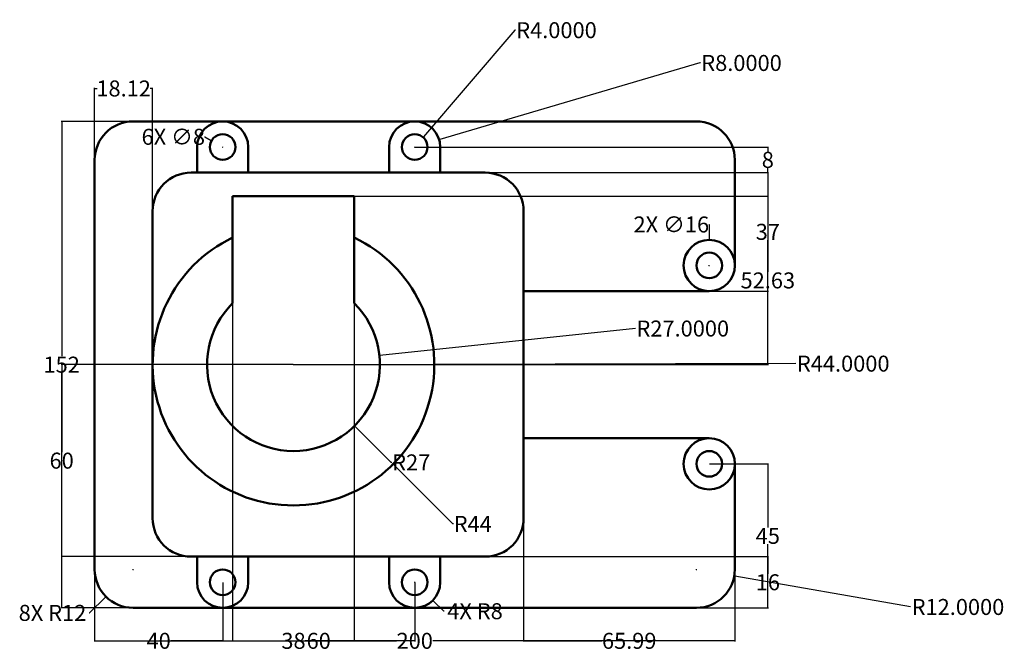
# Model space of a CAD drawing. Units: inches. Extents: x 381008 to 381315, y 259803 to 260000.
import ezdxf

# ---------------------------------------------------------------- set-up
doc = ezdxf.new("R2010")
doc.units = ezdxf.units.IN
doc.header["$MEASUREMENT"] = 0
doc.layers.add('M-DIMS', color=2, linetype='Continuous', lineweight=25)
doc.layers.add('M-OUTL', color=7, linetype='Continuous', lineweight=50)
doc.styles.get("Standard").update_dxf_attribs({"font": 'arial.ttf'})
doc.dimstyles.get("Standard").update_dxf_attribs({"dimtxt": 5, "dimasz": 0.18, "dimexe": 0.18, "dimexo": 0.0625, "dimgap": 0.09, "dimtad": 0, "dimtih": 1, "dimtoh": 1, "dimdec": 4, "dimzin": 0, "dimdsep": 46, "dimtxsty": 'Standard', "dimcen": 0.09, "dimadec": 0, "dimazin": 0, "dimtfac": 1, "dimtdec": 4, "dimtofl": 0, "dimtmove": 0, "dimatfit": 3, "dimfxl": 1, "dimtolj": 1, "dimtzin": 0, "dimarcsym": 0})

# ---------------------------------------------------------------- blocks, each defined once
blk = doc.blocks.new('*D1')
at = {"layer": 'Defpoints', "color": 0, "transparency": 16777216}
for p in [(381133.58, 259963.48), (381130.98, 259960.44)]:
    blk.add_point(p, dxfattribs=at)
at = {"layer": 'M-DIMS', "color": 0, "lineweight": -2, "transparency": 16777216}
for p, q in [((381162.25, 259996.96), (381133.7, 259963.62)), ((381162.43, 259996.96), (381162.25, 259996.96)), ((381130.89, 259960.44), (381131.07, 259960.44)), ((381130.98, 259960.35), (381130.98, 259960.53))]:
    blk.add_line(p, q, dxfattribs=at)
at = {"layer": 'M-DIMS', "color": 0, "transparency": 16777216}
blk.add_solid([(381133.68, 259963.64), (381133.72, 259963.6), (381133.58, 259963.48)], dxfattribs=at)
at = {"layer": 'M-DIMS', "color": 0, "transparency": 16777216, "insert": (381175.28, 259996.96), "char_height": 5, "attachment_point": 5}
blk.add_mtext('\\A1;R4.0000', dxfattribs=at)
blk = doc.blocks.new('*D2')
at = {"layer": 'Defpoints', "color": 0, "transparency": 16777216}
for p in [(381130.98, 259960.44), (381138.66, 259962.71)]:
    blk.add_point(p, dxfattribs=at)
at = {"layer": 'M-DIMS', "color": 0, "lineweight": -2, "transparency": 16777216}
for p, q in [((381220.06, 259986.72), (381138.83, 259962.76)), ((381220.24, 259986.72), (381220.06, 259986.72)), ((381130.89, 259960.44), (381131.07, 259960.44)), ((381130.98, 259960.35), (381130.98, 259960.53))]:
    blk.add_line(p, q, dxfattribs=at)
at = {"layer": 'M-DIMS', "color": 0, "transparency": 16777216}
blk.add_solid([(381138.82, 259962.79), (381138.84, 259962.73), (381138.66, 259962.71)], dxfattribs=at)
at = {"layer": 'M-DIMS', "color": 0, "transparency": 16777216, "insert": (381233.09, 259986.72), "char_height": 5, "attachment_point": 5}
blk.add_mtext('\\A1;R8.0000', dxfattribs=at)
blk = doc.blocks.new('*D3')
at = {"layer": 'Defpoints', "color": 0, "transparency": 16777216}
for p in [(381218.99, 259828.44), (381230.81, 259826.37)]:
    blk.add_point(p, dxfattribs=at)
at = {"layer": 'M-DIMS', "color": 0, "lineweight": -2, "transparency": 16777216}
for p, q in [((381218.9, 259828.44), (381219.08, 259828.44)), ((381218.99, 259828.35), (381218.99, 259828.53)), ((381285.92, 259816.72), (381230.98, 259826.34))]:
    blk.add_line(p, q, dxfattribs=at)
at = {"layer": 'M-DIMS', "color": 0, "transparency": 16777216}
blk.add_solid([(381230.99, 259826.37), (381230.98, 259826.31), (381230.81, 259826.37)], dxfattribs=at)
at = {"layer": 'M-DIMS', "color": 0, "transparency": 16777216, "insert": (381300.71, 259816.72), "char_height": 5, "attachment_point": 5}
blk.add_mtext('\\A1;R12.0000', dxfattribs=at)
blk = doc.blocks.new('*D4')
at = {"layer": 'Defpoints', "color": 0, "transparency": 16777216}
for p in [(381093.1, 259892.44), (381137.1, 259892.53)]:
    blk.add_point(p, dxfattribs=at)
at = {"layer": 'M-DIMS', "color": 0, "lineweight": -2, "transparency": 16777216}
for p, q in [((381250.06, 259892.76), (381137.28, 259892.53)), ((381093.01, 259892.44), (381093.19, 259892.44)), ((381093.1, 259892.35), (381093.1, 259892.53))]:
    blk.add_line(p, q, dxfattribs=at)
at = {"layer": 'M-DIMS', "color": 0, "transparency": 16777216}
blk.add_solid([(381137.28, 259892.56), (381137.28, 259892.5), (381137.1, 259892.53)], dxfattribs=at)
at = {"layer": 'M-DIMS', "color": 0, "transparency": 16777216, "insert": (381264.86, 259892.76), "char_height": 5, "attachment_point": 5}
blk.add_mtext('\\A1;R44.0000', dxfattribs=at)
blk = doc.blocks.new('*D5')
at = {"layer": 'Defpoints', "color": 0, "transparency": 16777216}
for p in [(381119.95, 259895.28), (381093.1, 259892.44)]:
    blk.add_point(p, dxfattribs=at)
at = {"layer": 'M-DIMS', "color": 0, "lineweight": -2, "transparency": 16777216}
for p, q in [((381199.94, 259903.73), (381120.13, 259895.3)), ((381093.01, 259892.44), (381093.19, 259892.44)), ((381093.1, 259892.35), (381093.1, 259892.53))]:
    blk.add_line(p, q, dxfattribs=at)
at = {"layer": 'M-DIMS', "color": 0, "transparency": 16777216}
blk.add_solid([(381120.13, 259895.33), (381120.13, 259895.27), (381119.95, 259895.28)], dxfattribs=at)
at = {"layer": 'M-DIMS', "color": 0, "transparency": 16777216, "insert": (381214.73, 259903.73), "char_height": 5, "attachment_point": 5}
blk.add_mtext('\\A1;R27.0000', dxfattribs=at)
blk = doc.blocks.new('MOUNTING-LUG')
for p, q in [((-8, 0), (-8, -8)), ((8, 0), (8, -8))]:
    blk.add_line(p, q)
blk.add_circle((0, 0), 4)
blk.add_arc((0, 0), 8, 0, 180)
blk = doc.blocks.new('CONCENTRIC-MOUNT-HOLE')
for radius in [8, 4]:
    blk.add_circle((0, 0), radius)
blk = doc.blocks.new('*D8')
at = {"layer": 'Defpoints', "color": 0, "transparency": 16777216}
for p in [(381030.98, 259828.44), (381230.99, 259828.44), (381230.99, 259806.14)]:
    blk.add_point(p, dxfattribs=at)
at = {"layer": 'M-DIMS', "color": 0, "lineweight": -2, "transparency": 16777216}
for p, q in [((381030.98, 259828.38), (381030.98, 259805.96)), ((381230.99, 259828.38), (381230.99, 259805.96)), ((381031.16, 259806.14), (381125.34, 259806.14)), ((381230.81, 259806.14), (381136.63, 259806.14))]:
    blk.add_line(p, q, dxfattribs=at)
at = {"layer": 'M-DIMS', "color": 0, "transparency": 16777216}
for points in [[(381031.16, 259806.17), (381031.16, 259806.11), (381030.98, 259806.14)], [(381230.81, 259806.17), (381230.81, 259806.11), (381230.99, 259806.14)]]:
    blk.add_solid(points, dxfattribs=at)
at = {"layer": 'M-DIMS', "color": 0, "transparency": 16777216, "insert": (381130.98, 259806.14), "char_height": 5, "attachment_point": 5}
blk.add_mtext('\\A1;200', dxfattribs=at)
blk = doc.blocks.new('*D9')
at = {"layer": 'Defpoints', "color": 0, "transparency": 16777216}
for p in [(381020.68, 259968.44), (381042.98, 259968.44), (381042.98, 259816.44)]:
    blk.add_point(p, dxfattribs=at)
at = {"layer": 'M-DIMS', "color": 0, "lineweight": -2, "transparency": 16777216}
for p, q in [((381042.92, 259968.44), (381020.5, 259968.44)), ((381020.68, 259968.26), (381020.68, 259895.09)), ((381020.68, 259816.62), (381020.68, 259889.8)), ((381042.92, 259816.44), (381020.5, 259816.44))]:
    blk.add_line(p, q, dxfattribs=at)
at = {"layer": 'M-DIMS', "color": 0, "transparency": 16777216}
for points in [[(381020.65, 259968.26), (381020.71, 259968.26), (381020.68, 259968.44)], [(381020.65, 259816.62), (381020.71, 259816.62), (381020.68, 259816.44)]]:
    blk.add_solid(points, dxfattribs=at)
at = {"layer": 'M-DIMS', "color": 0, "transparency": 16777216, "insert": (381020.68, 259892.44), "char_height": 5, "attachment_point": 5}
blk.add_mtext('\\A1;152', dxfattribs=at)
blk = doc.blocks.new('*D10')
at = {"layer": 'Defpoints', "color": 0, "transparency": 16777216}
for p in [(381030.98, 259828.44), (381070.98, 259824.44), (381070.98, 259806.14)]:
    blk.add_point(p, dxfattribs=at)
at = {"layer": 'M-DIMS', "color": 0, "lineweight": -2, "transparency": 16777216}
for p, q in [((381030.98, 259828.38), (381030.98, 259805.96)), ((381070.98, 259824.38), (381070.98, 259805.96)), ((381031.16, 259806.14), (381047.22, 259806.14)), ((381070.8, 259806.14), (381054.75, 259806.14))]:
    blk.add_line(p, q, dxfattribs=at)
at = {"layer": 'M-DIMS', "color": 0, "transparency": 16777216}
for points in [[(381031.16, 259806.17), (381031.16, 259806.11), (381030.98, 259806.14)], [(381070.8, 259806.17), (381070.8, 259806.11), (381070.98, 259806.14)]]:
    blk.add_solid(points, dxfattribs=at)
at = {"layer": 'M-DIMS', "color": 0, "transparency": 16777216, "insert": (381050.98, 259806.14), "char_height": 5, "attachment_point": 5}
blk.add_mtext('\\A1;40', dxfattribs=at)
blk = doc.blocks.new('*D11')
at = {"layer": 'Defpoints', "color": 0, "transparency": 16777216}
for p in [(381070.98, 259824.44), (381130.98, 259824.44), (381130.98, 259806.14)]:
    blk.add_point(p, dxfattribs=at)
at = {"layer": 'M-DIMS', "color": 0, "lineweight": -2, "transparency": 16777216}
for p, q in [((381070.98, 259824.38), (381070.98, 259805.96)), ((381130.98, 259824.38), (381130.98, 259805.96)), ((381071.16, 259806.14), (381097.31, 259806.14)), ((381130.8, 259806.14), (381104.66, 259806.14))]:
    blk.add_line(p, q, dxfattribs=at)
at = {"layer": 'M-DIMS', "color": 0, "transparency": 16777216}
for points in [[(381071.16, 259806.17), (381071.16, 259806.11), (381070.98, 259806.14)], [(381130.8, 259806.17), (381130.8, 259806.11), (381130.98, 259806.14)]]:
    blk.add_solid(points, dxfattribs=at)
at = {"layer": 'M-DIMS', "color": 0, "transparency": 16777216, "insert": (381100.98, 259806.14), "char_height": 5, "attachment_point": 5}
blk.add_mtext('\\A1;60', dxfattribs=at)
blk = doc.blocks.new('*D12')
at = {"layer": 'Defpoints', "color": 0, "transparency": 16777216}
for p in [(381049.1, 259978.74), (381030.98, 259956.44), (381049.1, 259940.44)]:
    blk.add_point(p, dxfattribs=at)
at = {"layer": 'M-DIMS', "color": 0, "lineweight": -2, "transparency": 16777216}
for p, q in [((381030.98, 259956.51), (381030.98, 259978.92)), ((381049.1, 259940.51), (381049.1, 259978.92)), ((381031.16, 259978.74), (381031.78, 259978.74)), ((381048.92, 259978.74), (381048.31, 259978.74))]:
    blk.add_line(p, q, dxfattribs=at)
at = {"layer": 'M-DIMS', "color": 0, "transparency": 16777216}
for points in [[(381031.16, 259978.77), (381031.16, 259978.71), (381030.98, 259978.74)], [(381048.92, 259978.77), (381048.92, 259978.71), (381049.1, 259978.74)]]:
    blk.add_solid(points, dxfattribs=at)
at = {"layer": 'M-DIMS', "color": 0, "transparency": 16777216, "insert": (381040.04, 259978.74), "char_height": 5, "attachment_point": 5}
blk.add_mtext('\\A1;18.12', dxfattribs=at)
blk = doc.blocks.new('*D13')
at = {"layer": 'Defpoints', "color": 0, "transparency": 16777216}
for p in [(381165, 259844.44), (381230.99, 259828.44), (381230.99, 259806.14)]:
    blk.add_point(p, dxfattribs=at)
at = {"layer": 'M-DIMS', "color": 0, "lineweight": -2, "transparency": 16777216}
for p, q in [((381165, 259844.38), (381165, 259805.96)), ((381230.99, 259828.38), (381230.99, 259805.96)), ((381165.18, 259806.14), (381189.45, 259806.14)), ((381230.81, 259806.14), (381206.54, 259806.14))]:
    blk.add_line(p, q, dxfattribs=at)
at = {"layer": 'M-DIMS', "color": 0, "transparency": 16777216}
for points in [[(381165.18, 259806.17), (381165.18, 259806.11), (381165, 259806.14)], [(381230.81, 259806.17), (381230.81, 259806.11), (381230.99, 259806.14)]]:
    blk.add_solid(points, dxfattribs=at)
at = {"layer": 'M-DIMS', "color": 0, "transparency": 16777216, "insert": (381197.99, 259806.14), "char_height": 5, "attachment_point": 5}
blk.add_mtext('\\A1;65.99', dxfattribs=at)
blk = doc.blocks.new('*D14')
at = {"layer": 'Defpoints', "color": 0, "transparency": 16777216}
for p in [(381020.68, 259892.44), (381093.1, 259892.44), (381061.1, 259832.44)]:
    blk.add_point(p, dxfattribs=at)
at = {"layer": 'M-DIMS', "color": 0, "lineweight": -2, "transparency": 16777216}
for p, q in [((381093.04, 259892.44), (381020.5, 259892.44)), ((381020.68, 259892.26), (381020.68, 259865.09)), ((381020.68, 259832.62), (381020.68, 259859.8)), ((381061.04, 259832.44), (381020.5, 259832.44))]:
    blk.add_line(p, q, dxfattribs=at)
at = {"layer": 'M-DIMS', "color": 0, "transparency": 16777216}
for points in [[(381020.65, 259892.26), (381020.71, 259892.26), (381020.68, 259892.44)], [(381020.65, 259832.62), (381020.71, 259832.62), (381020.68, 259832.44)]]:
    blk.add_solid(points, dxfattribs=at)
at = {"layer": 'M-DIMS', "color": 0, "transparency": 16777216, "insert": (381020.68, 259862.44), "char_height": 5, "attachment_point": 5}
blk.add_mtext('\\A1;60', dxfattribs=at)
blk = doc.blocks.new('*D15')
at = {"layer": 'Defpoints', "color": 0, "transparency": 16777216}
for p in [(381130.98, 259960.44), (381153, 259952.44), (381241.3, 259952.44)]:
    blk.add_point(p, dxfattribs=at)
at = {"layer": 'M-DIMS', "color": 0, "lineweight": -2, "transparency": 16777216}
for p, q in [((381131.04, 259960.44), (381241.48, 259960.44)), ((381241.3, 259960.26), (381241.3, 259959.09)), ((381153.06, 259952.44), (381241.48, 259952.44)), ((381241.3, 259952.62), (381241.3, 259953.8))]:
    blk.add_line(p, q, dxfattribs=at)
at = {"layer": 'M-DIMS', "color": 0, "transparency": 16777216}
for points in [[(381241.27, 259960.26), (381241.33, 259960.26), (381241.3, 259960.44)], [(381241.27, 259952.62), (381241.33, 259952.62), (381241.3, 259952.44)]]:
    blk.add_solid(points, dxfattribs=at)
at = {"layer": 'M-DIMS', "color": 0, "transparency": 16777216, "insert": (381241.3, 259956.44), "char_height": 5, "attachment_point": 5}
blk.add_mtext('\\A1;8', dxfattribs=at)
blk = doc.blocks.new('*D16')
at = {"layer": 'Defpoints', "color": 0, "transparency": 16777216}
for p in [(381153, 259832.44), (381241.3, 259832.44), (381218.99, 259816.44)]:
    blk.add_point(p, dxfattribs=at)
at = {"layer": 'M-DIMS', "color": 0, "lineweight": -2, "transparency": 16777216}
for p, q in [((381153.06, 259832.44), (381241.48, 259832.44)), ((381241.3, 259832.26), (381241.3, 259827.09)), ((381241.3, 259816.62), (381241.3, 259821.8)), ((381219.05, 259816.44), (381241.48, 259816.44))]:
    blk.add_line(p, q, dxfattribs=at)
at = {"layer": 'M-DIMS', "color": 0, "transparency": 16777216}
for points in [[(381241.27, 259832.26), (381241.33, 259832.26), (381241.3, 259832.44)], [(381241.27, 259816.62), (381241.33, 259816.62), (381241.3, 259816.44)]]:
    blk.add_solid(points, dxfattribs=at)
at = {"layer": 'M-DIMS', "color": 0, "transparency": 16777216, "insert": (381241.3, 259824.44), "char_height": 5, "attachment_point": 5}
blk.add_mtext('\\A1;16', dxfattribs=at)
blk = doc.blocks.new('*D17')
at = {"layer": 'Defpoints', "color": 0, "transparency": 16777216}
for p in [(381153, 259952.44), (381241.3, 259952.44), (381165, 259915.44)]:
    blk.add_point(p, dxfattribs=at)
at = {"layer": 'M-DIMS', "color": 0, "lineweight": -2, "transparency": 16777216}
for p, q in [((381153.06, 259952.44), (381241.48, 259952.44)), ((381241.3, 259952.26), (381241.3, 259936.59)), ((381241.3, 259915.62), (381241.3, 259931.3)), ((381165.06, 259915.44), (381241.48, 259915.44))]:
    blk.add_line(p, q, dxfattribs=at)
at = {"layer": 'M-DIMS', "color": 0, "transparency": 16777216}
for points in [[(381241.27, 259952.26), (381241.33, 259952.26), (381241.3, 259952.44)], [(381241.27, 259915.62), (381241.33, 259915.62), (381241.3, 259915.44)]]:
    blk.add_solid(points, dxfattribs=at)
at = {"layer": 'M-DIMS', "color": 0, "transparency": 16777216, "insert": (381241.3, 259933.94), "char_height": 5, "attachment_point": 5}
blk.add_mtext('\\A1;37', dxfattribs=at)
blk = doc.blocks.new('*D18')
at = {"layer": 'Defpoints', "color": 0, "transparency": 16777216}
for p in [(381223.000594, 259861.442622), (381241.300594, 259861.442622), (381218.986961, 259816.442622)]:
    blk.add_point(p, dxfattribs=at)
at = {"layer": 'M-DIMS', "color": 0, "lineweight": -2, "transparency": 16777216}
for p, q in [((381223.063094, 259861.442622), (381241.480594, 259861.442622)), ((381241.300594, 259861.262622), (381241.300594, 259841.575255)), ((381241.300594, 259816.622622), (381241.300594, 259836.309989)), ((381219.049461, 259816.442622), (381241.480594, 259816.442622))]:
    blk.add_line(p, q, dxfattribs=at)
at = {"layer": 'M-DIMS', "color": 0, "transparency": 16777216}
for points in [[(381241.270594, 259861.262622), (381241.330594, 259861.262622), (381241.300594, 259861.442622)], [(381241.270594, 259816.622622), (381241.330594, 259816.622622), (381241.300594, 259816.442622)]]:
    blk.add_solid(points, dxfattribs=at)
at = {"layer": 'M-DIMS', "color": 0, "transparency": 16777216, "insert": (381241.300594, 259838.942622), "char_height": 5, "attachment_point": 5}
blk.add_mtext('\\A1;45', dxfattribs=at)
blk = doc.blocks.new('*D19')
at = {"layer": 'Defpoints', "color": 0, "transparency": 16777216}
for p in [(381074.1, 259945.07), (381112.1, 259945.07), (381112.1, 259806.14)]:
    blk.add_point(p, dxfattribs=at)
at = {"layer": 'M-DIMS', "color": 0, "lineweight": -2, "transparency": 16777216}
for p, q in [((381074.1, 259945.01), (381074.1, 259805.96)), ((381112.1, 259945.01), (381112.1, 259805.96)), ((381074.28, 259806.14), (381089.43, 259806.14)), ((381111.92, 259806.14), (381096.77, 259806.14))]:
    blk.add_line(p, q, dxfattribs=at)
at = {"layer": 'M-DIMS', "color": 0, "transparency": 16777216}
for points in [[(381074.28, 259806.17), (381074.28, 259806.11), (381074.1, 259806.14)], [(381111.92, 259806.17), (381111.92, 259806.11), (381112.1, 259806.14)]]:
    blk.add_solid(points, dxfattribs=at)
at = {"layer": 'M-DIMS', "color": 0, "transparency": 16777216, "insert": (381093.1, 259806.14), "char_height": 5, "attachment_point": 5}
blk.add_mtext('\\A1;38', dxfattribs=at)
blk = doc.blocks.new('*D20')
at = {"layer": 'Defpoints', "color": 0, "transparency": 16777216}
for p in [(381112.1, 259945.07), (381241.3, 259945.07), (381093.1, 259892.44)]:
    blk.add_point(p, dxfattribs=at)
at = {"layer": 'M-DIMS', "color": 0, "lineweight": -2, "transparency": 16777216}
for p, q in [((381112.16, 259945.07), (381241.48, 259945.07)), ((381241.3, 259944.89), (381241.3, 259921.4)), ((381241.3, 259892.62), (381241.3, 259916.11)), ((381093.16, 259892.44), (381241.48, 259892.44))]:
    blk.add_line(p, q, dxfattribs=at)
at = {"layer": 'M-DIMS', "color": 0, "transparency": 16777216}
for points in [[(381241.27, 259944.89), (381241.33, 259944.89), (381241.3, 259945.07)], [(381241.27, 259892.62), (381241.33, 259892.62), (381241.3, 259892.44)]]:
    blk.add_solid(points, dxfattribs=at)
at = {"layer": 'M-DIMS', "color": 0, "transparency": 16777216, "insert": (381241.3, 259918.76), "char_height": 5, "attachment_point": 5}
blk.add_mtext('\\A1;52.63', dxfattribs=at)
blk = doc.blocks.new('*D21')
at = {"layer": 'Defpoints', "color": 0, "transparency": 16777216}
for p in [(381042.98, 259828.44), (381034.5, 259819.96)]:
    blk.add_point(p, dxfattribs=at)
at = {"layer": 'M-DIMS', "color": 0, "lineweight": -2, "transparency": 16777216}
for p, q in [((381042.89, 259828.44), (381043.07, 259828.44)), ((381042.98, 259828.35), (381042.98, 259828.53)), ((381029.41, 259814.87), (381034.37, 259819.83)), ((381029.23, 259814.87), (381029.41, 259814.87))]:
    blk.add_line(p, q, dxfattribs=at)
at = {"layer": 'M-DIMS', "color": 0, "transparency": 16777216}
blk.add_solid([(381034.35, 259819.85), (381034.39, 259819.81), (381034.5, 259819.96)], dxfattribs=at)
at = {"layer": 'M-DIMS', "color": 0, "transparency": 16777216, "insert": (381017.81, 259814.87), "char_height": 5, "attachment_point": 5}
blk.add_mtext('\\A1;8X R12', dxfattribs=at)
blk = doc.blocks.new('*D22')
at = {"layer": 'Defpoints', "color": 0, "transparency": 16777216}
for p in [(381130.98, 259824.44), (381136.64, 259818.79)]:
    blk.add_point(p, dxfattribs=at)
at = {"layer": 'M-DIMS', "color": 0, "lineweight": -2, "transparency": 16777216}
for p, q in [((381130.89, 259824.44), (381131.07, 259824.44)), ((381130.98, 259824.35), (381130.98, 259824.53)), ((381140.04, 259815.4), (381136.77, 259818.66)), ((381140.22, 259815.4), (381140.04, 259815.4))]:
    blk.add_line(p, q, dxfattribs=at)
at = {"layer": 'M-DIMS', "color": 0, "transparency": 16777216}
blk.add_solid([(381136.79, 259818.68), (381136.75, 259818.64), (381136.64, 259818.79)], dxfattribs=at)
at = {"layer": 'M-DIMS', "color": 0, "transparency": 16777216, "insert": (381149.82, 259815.4), "char_height": 5, "attachment_point": 5}
blk.add_mtext('\\A1;4X R8', dxfattribs=at)
blk = doc.blocks.new('*D23')
at = {"layer": 'Defpoints', "color": 0, "transparency": 16777216}
for p in [(381067.52, 259962.44), (381074.45, 259958.44)]:
    blk.add_point(p, dxfattribs=at)
at = {"layer": 'M-DIMS', "color": 0, "lineweight": -2, "transparency": 16777216}
for p, q in [((381065.26, 259963.64), (381065.44, 259963.64)), ((381065.44, 259963.64), (381067.36, 259962.53)), ((381070.89, 259960.44), (381071.07, 259960.44)), ((381070.98, 259960.35), (381070.98, 259960.53))]:
    blk.add_line(p, q, dxfattribs=at)
at = {"layer": 'M-DIMS', "color": 0, "transparency": 16777216}
blk.add_solid([(381067.38, 259962.56), (381067.35, 259962.51), (381067.52, 259962.44)], dxfattribs=at)
at = {"layer": 'M-DIMS', "color": 0, "transparency": 16777216, "insert": (381055.55, 259963.64), "char_height": 5, "attachment_point": 5}
blk.add_mtext('\\A1;6X ∅8', dxfattribs=at)
blk = doc.blocks.new('*D24')
at = {"layer": 'Defpoints', "color": 0, "transparency": 16777216}
for p in [(381223, 259931.44), (381223, 259915.44)]:
    blk.add_point(p, dxfattribs=at)
at = {"layer": 'M-DIMS', "color": 0, "lineweight": -2, "transparency": 16777216}
for p, q in [((381222.82, 259936.24), (381223, 259936.24)), ((381223, 259936.24), (381223, 259931.62)), ((381222.91, 259923.44), (381223.09, 259923.44)), ((381223, 259923.35), (381223, 259923.53))]:
    blk.add_line(p, q, dxfattribs=at)
at = {"layer": 'M-DIMS', "color": 0, "transparency": 16777216}
blk.add_solid([(381223.03, 259931.62), (381222.97, 259931.62), (381223, 259931.44)], dxfattribs=at)
at = {"layer": 'M-DIMS', "color": 0, "transparency": 16777216, "insert": (381211.15, 259936.24), "char_height": 5, "attachment_point": 5}
blk.add_mtext('\\A1;2X ∅16', dxfattribs=at)
blk = doc.blocks.new('*D25')
at = {"layer": 'Defpoints', "color": 0, "transparency": 16777216}
for p in [(381093.1, 259892.44), (381112.19, 259873.35)]:
    blk.add_point(p, dxfattribs=at)
at = {"layer": 'M-DIMS', "color": 0, "lineweight": -2, "transparency": 16777216}
for p, q in [((381093.01, 259892.44), (381093.19, 259892.44)), ((381093.1, 259892.35), (381093.1, 259892.53)), ((381123.64, 259861.89), (381112.32, 259873.22)), ((381123.82, 259861.89), (381123.64, 259861.89))]:
    blk.add_line(p, q, dxfattribs=at)
at = {"layer": 'M-DIMS', "color": 0, "transparency": 16777216}
blk.add_solid([(381112.34, 259873.24), (381112.3, 259873.2), (381112.19, 259873.35)], dxfattribs=at)
at = {"layer": 'M-DIMS', "color": 0, "transparency": 16777216, "insert": (381129.89, 259861.89), "char_height": 5, "attachment_point": 5}
blk.add_mtext('\\A1;R27', dxfattribs=at)
blk = doc.blocks.new('*D26')
at = {"layer": 'Defpoints', "color": 0, "transparency": 16777216}
for p in [(381093.1, 259892.44), (381124.22, 259861.33)]:
    blk.add_point(p, dxfattribs=at)
at = {"layer": 'M-DIMS', "color": 0, "lineweight": -2, "transparency": 16777216}
for p, q in [((381093.01, 259892.44), (381093.19, 259892.44)), ((381093.1, 259892.35), (381093.1, 259892.53)), ((381142.89, 259842.67), (381124.34, 259861.21)), ((381143.07, 259842.67), (381142.89, 259842.67))]:
    blk.add_line(p, q, dxfattribs=at)
at = {"layer": 'M-DIMS', "color": 0, "transparency": 16777216}
blk.add_solid([(381124.37, 259861.23), (381124.32, 259861.18), (381124.22, 259861.33)], dxfattribs=at)
at = {"layer": 'M-DIMS', "color": 0, "transparency": 16777216, "insert": (381149.12, 259842.67), "char_height": 5, "attachment_point": 5}
blk.add_mtext('\\A1;R44', dxfattribs=at)

msp = doc.modelspace()

# ---------------------------------------------------------------- linework, layer by layer
at = {"layer": 'M-OUTL'}
for p, q in [((381042.982, 259968.44262), (381070.982, 259968.44262)), ((381070.982, 259968.44262), (381130.982, 259968.44262)), ((381130.982, 259968.44262), (381218.98696, 259968.44262)), ((381030.982, 259956.44262), (381030.982, 259828.44262)), ((381230.98696, 259956.44758), (381231.00059, 259923.44262)), ((381070.982, 259952.44262), (381061.10027, 259952.44262)), ((381070.982, 259952.44262), (381153.00059, 259952.44262)), ((381074.10027, 259911.62595), (381074.10027, 259945.07301)), ((381074.10027, 259945.07301), (381112.10027, 259945.07301)), ((381112.10027, 259911.62595), (381112.10027, 259945.07301)), ((381049.10027, 259940.44262), (381049.10027, 259844.44262)), ((381165.00059, 259940.44262), (381165.00059, 259844.44262)), ((381223.00059, 259915.44262), (381165.00059, 259915.44262)), ((381223.00059, 259869.44262), (381165.00059, 259869.44262)), ((381230.98696, 259828.43767), (381231.00059, 259861.44262)), ((381070.982, 259832.44262), (381061.10027, 259832.44262)), ((381070.982, 259832.44262), (381153.00059, 259832.44262)), ((381042.982, 259816.44262), (381218.98696, 259816.44262))]:
    msp.add_line(p, q, dxfattribs=at)
for centre, radius, start, end in [((381042.982, 259956.44262), 12, 90, 180), ((381218.98696, 259956.44262), 12, 0.0236683, 90), ((381061.10027, 259940.44262), 12, 90, 180), ((381153.00059, 259940.44262), 12, 0, 90), ((381093.10027, 259892.44262), 44, 115.583002, 64.416998), ((381093.10027, 259892.44262), 27, 134.7249132, 45.2750868), ((381061.10027, 259844.44262), 12, 180, 270), ((381153.00059, 259844.44262), 12, 270, 0), ((381042.982, 259828.44262), 12, 180, 270), ((381218.98696, 259828.44262), 12, 270, 359.9763317)]:
    msp.add_arc(centre, radius, start, end, dxfattribs=at)

# ---------------------------------------------------------------- block references
for name, p in [('MOUNTING-LUG', (381070.982, 259960.44262)), ('MOUNTING-LUG', (381130.982, 259960.44262)), ('CONCENTRIC-MOUNT-HOLE', (381223.00059, 259923.44262)), ('CONCENTRIC-MOUNT-HOLE', (381223.00059, 259861.44262))]:
    msp.add_blockref(name, p, dxfattribs=at)
at = {"layer": 'M-OUTL', "rotation": 180}
for p in [(381070.982, 259824.44262), (381130.982, 259824.44262)]:
    msp.add_blockref('MOUNTING-LUG', p, dxfattribs=at)

# ---------------------------------------------------------------- dimensions: what is measured, and where the dimension line sits
at = {"layer": 'M-DIMS'}
for center, mpoint, override, picture, middle in [((381130.982, 259960.44262), (381133.58385, 259963.48078), {"dimclrd": 0, "dimclre": 0, "dimclrt": 0}, '*D1', (381175.28458, 259996.9563)), ((381130.982, 259960.44262), (381138.65513, 259962.70605), {"dimclrd": 0, "dimclre": 0, "dimclrt": 0}, '*D2', (381233.09337, 259986.71914)), ((381093.10027, 259892.44262), (381119.95079, 259895.2798), {"dimclrd": 0, "dimclre": 0, "dimclrt": 0}, '*D5', (381199.93713, 259903.73159)), ((381093.10027, 259892.44262), (381137.10017, 259892.53286), {"dimclrd": 0, "dimclre": 0, "dimclrt": 0}, '*D4', (381250.06257, 259892.76452)), ((381093.10027, 259892.44262), (381112.19071, 259873.34929), {"dimdec": 0, "dimlfac": 1, "dimrnd": 0, "dimzin": 0, "dimdsep": 46, "dimlunit": 2}, '*D25', (381129.88871, 259861.8933)), ((381093.10027, 259892.44262), (381124.21652, 259861.33348), {"dimdec": 0, "dimlfac": 1, "dimrnd": 0, "dimzin": 0, "dimdsep": 46, "dimlunit": 2}, '*D26', (381149.11978, 259842.66799)), ((381218.98696, 259828.44262), (381230.80711, 259826.37283), {"dimclrd": 0, "dimclre": 0, "dimclrt": 0}, '*D3', (381285.91725, 259816.72263))]:
    dim = msp.add_radius_dim(center=center, mpoint=mpoint, dimstyle='Standard', override=override, dxfattribs=at)
    dim.commit()
    dim.dimension.update_dxf_attribs({"geometry": picture, "text_midpoint": middle, "dimtype": 164})
for base, p1, p2, override, picture, middle in [((381049.10027, 259978.74262), (381030.982, 259956.44262), (381049.10027, 259940.44262), {"dimdec": 2, "dimlfac": 1, "dimrnd": 0, "dimzin": 0, "dimdsep": 46, "dimlunit": 2}, '*D12', (381040.04114, 259978.74262)), ((381112.10027, 259806.14262), (381074.10027, 259945.07301), (381112.10027, 259945.07301), {"dimdec": 0, "dimlfac": 1, "dimrnd": 0, "dimzin": 0, "dimdsep": 46, "dimlunit": 2}, '*D19', (381093.10027, 259806.14262)), ((381230.98696, 259806.14262), (381165.00059, 259844.44262), (381230.98696, 259828.43767), {"dimdec": 2, "dimlfac": 1, "dimrnd": 0, "dimzin": 0, "dimdsep": 46, "dimlunit": 2}, '*D13', (381197.99378, 259806.14262)), ((381230.98696, 259806.14262), (381030.982, 259828.44262), (381230.98696, 259828.43767), {"dimdec": 0, "dimlfac": 1, "dimrnd": 0, "dimzin": 0, "dimdsep": 46, "dimlunit": 2}, '*D8', (381130.98448, 259806.14262)), ((381070.982, 259806.14262), (381030.982, 259828.44262), (381070.982, 259824.44262), {"dimdec": 0, "dimlfac": 1, "dimrnd": 0, "dimzin": 0, "dimdsep": 46, "dimlunit": 2}, '*D10', (381050.982, 259806.14262)), ((381130.98201, 259806.14262), (381070.982, 259824.44262), (381130.98201, 259824.44262), {"dimdec": 0, "dimlfac": 1, "dimrnd": 0, "dimzin": 0, "dimdsep": 46, "dimlunit": 2}, '*D11', (381100.98201, 259806.14262))]:
    dim = msp.add_linear_dim(base=base, p1=p1, p2=p2, dimstyle='Standard', override=override, dxfattribs=at)
    dim.commit()
    dim.dimension.update_dxf_attribs({"geometry": picture, "text_midpoint": middle})
for p1, p2, text, picture, middle in [((381074.44542, 259958.44143), (381067.51859, 259962.44381), '6X <>', '*D23', (381055.55424, 259963.64453)), ((381223.00119, 259915.44262), (381223, 259931.44262), '2X <>', '*D24', (381211.14881, 259936.24262))]:
    dim = msp.add_diameter_dim_2p(p1=p1, p2=p2, text=text, dimstyle='Standard', override={"dimdec": 0, "dimlfac": 1, "dimrnd": 0, "dimzin": 0, "dimdsep": 46, "dimlunit": 2}, dxfattribs=at)
    dim.commit()
    dim.dimension.update_dxf_attribs({"geometry": picture, "text_midpoint": middle, "dimtype": 163})
for base, p1, p2, override, picture, middle in [((381020.68201, 259968.44262), (381042.982, 259816.44262), (381042.982, 259968.44262), {"dimdec": 0, "dimlfac": 1, "dimrnd": 0, "dimzin": 0, "dimdsep": 46, "dimlunit": 2}, '*D9', (381020.68201, 259892.44262)), ((381241.30059, 259952.44262), (381130.98201, 259960.44262), (381153.00059, 259952.44262), {"dimdec": 0, "dimlfac": 1, "dimrnd": 0, "dimzin": 0, "dimdsep": 46, "dimlunit": 2}, '*D15', (381241.30059, 259956.44262)), ((381241.30059, 259952.44262), (381165.00059, 259915.44262), (381153.00059, 259952.44262), {"dimdec": 0, "dimlfac": 1, "dimrnd": 0, "dimzin": 0, "dimdsep": 46, "dimlunit": 2}, '*D17', (381241.30059, 259933.94262)), ((381241.30059, 259945.07301), (381093.10027, 259892.44262), (381112.10027, 259945.07301), {"dimdec": 2, "dimlfac": 1, "dimrnd": 0, "dimzin": 0, "dimdsep": 46, "dimlunit": 2}, '*D20', (381241.30059, 259918.75782)), ((381020.68201, 259892.44262), (381061.10027, 259832.44262), (381093.10027, 259892.44262), {"dimdec": 0, "dimlfac": 1, "dimrnd": 0, "dimzin": 0, "dimdsep": 46, "dimlunit": 2}, '*D14', (381020.68201, 259862.44262)), ((381241.30059, 259861.44262), (381218.98696, 259816.44262), (381223.00059, 259861.44262), {"dimdec": 0, "dimlfac": 1, "dimrnd": 0, "dimzin": 0, "dimdsep": 46, "dimlunit": 2}, '*D18', (381241.30059, 259838.94262)), ((381241.30059, 259832.44262), (381218.98696, 259816.44262), (381153.00059, 259832.44262), {"dimdec": 0, "dimlfac": 1, "dimrnd": 0, "dimzin": 0, "dimdsep": 46, "dimlunit": 2}, '*D16', (381241.30059, 259824.44262))]:
    dim = msp.add_linear_dim(base=base, p1=p1, p2=p2, angle=90, dimstyle='Standard', override=override, dxfattribs=at)
    dim.commit()
    dim.dimension.update_dxf_attribs({"geometry": picture, "text_midpoint": middle})
for center, mpoint, text, picture, middle in [((381042.982, 259828.44262), (381034.49703, 259819.95703), '8X <>', '*D21', (381017.81272, 259814.86568)), ((381130.98201, 259824.44262), (381136.64155, 259818.78846), '4X <>', '*D22', (381149.81614, 259815.39596))]:
    dim = msp.add_radius_dim(center=center, mpoint=mpoint, text=text, dimstyle='Standard', override={"dimdec": 0, "dimlfac": 1, "dimrnd": 0, "dimzin": 0, "dimdsep": 46, "dimlunit": 2}, dxfattribs=at)
    dim.commit()
    dim.dimension.update_dxf_attribs({"geometry": picture, "text_midpoint": middle, "dimtype": 164})

doc.saveas('drawing.dxf')
